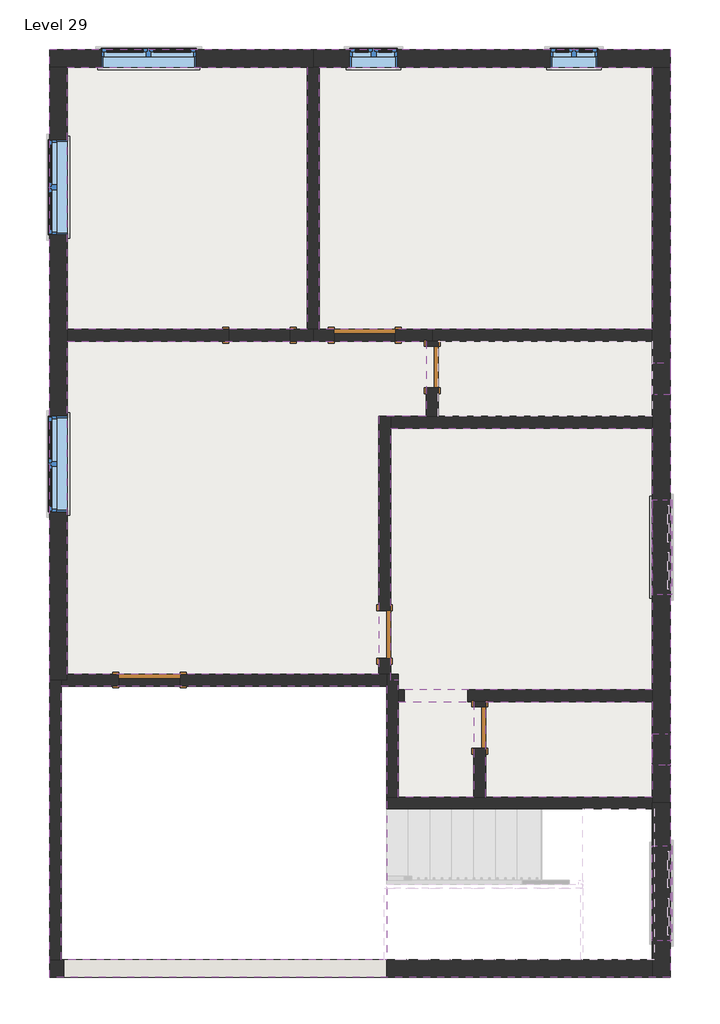
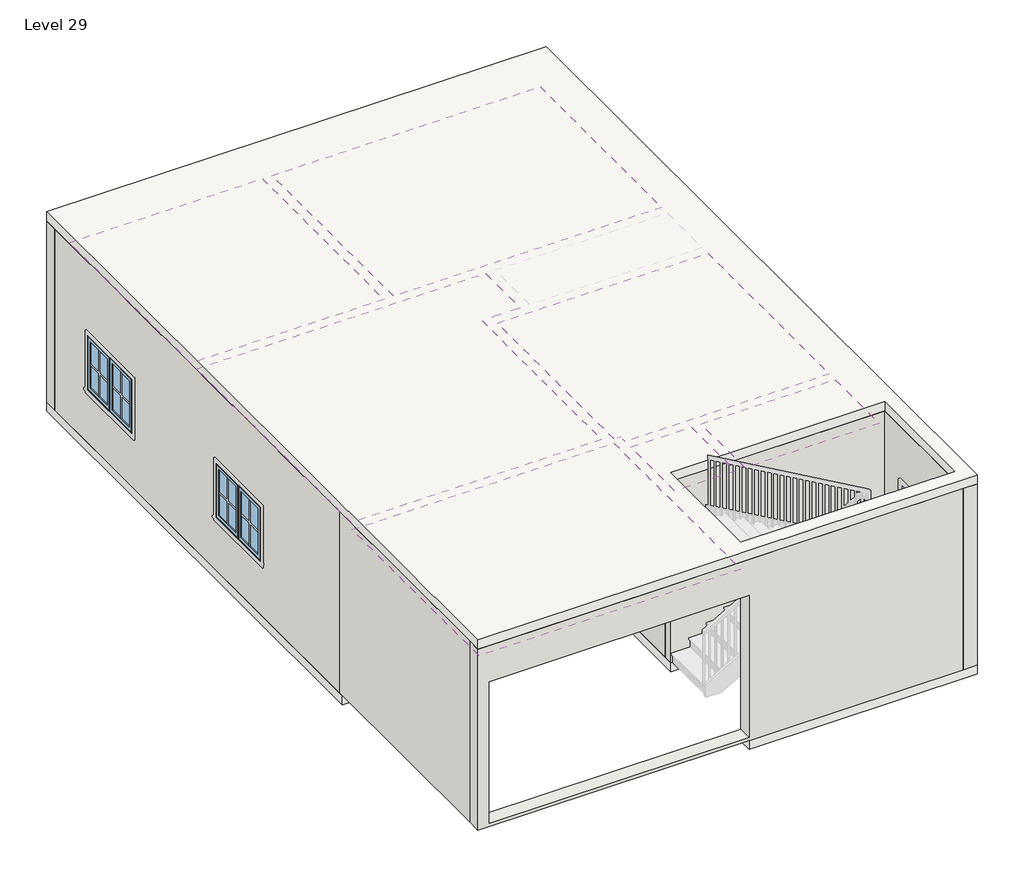
# One storey, part 1 of 2: 27 walls, 13 windows, 7 coverings, 6 doors, 2 slabs.
# Revit data of these elements (continued)
# Element 48 (IfcWindow, "Window-Casement-Double : 3'") (continued)
#   Frame Extension = 0' - 0 1/4"
#   Exterior Wall Closure = 0' - 1 1/4"
#   Interior Trim Visibility = yes
#   Exterior Trim Visibility = yes
#   Phase Created = New Construction
#   Materials on its faces: "Wood - Stained", "Glass", "Clad - White"
# Element 49 (IfcWindow, "Window-Casement-Double : 4'")
#   Mark = "131"
#   Window Inset = 0' - 0"
#   Interior Wall Closure = 0' - 2 1/4"
#   Frame Extension = 0' - 0 1/4"
#   Exterior Wall Closure = 0' - 1 1/4"
#   Interior Trim Visibility = yes
#   Exterior Trim Visibility = yes
#   Phase Created = New Construction
#   Materials on its faces: "Wood - Stained", "Glass", "Clad - White"
# Element 50 (IfcWindow, "Window-Casement-Double : 4'")
#   Mark = "132"
#   Window Inset = 0' - 0"
#   Interior Wall Closure = 0' - 2 1/4"
#   Frame Extension = 0' - 0 1/4"
#   Exterior Wall Closure = 0' - 1 1/4"
#   Interior Trim Visibility = yes
#   Exterior Trim Visibility = yes
#   Phase Created = New Construction
#   Materials on its faces: "Wood - Stained", "Glass", "Clad - White"
# Element 51 (IfcWindow, "Window-Casement-Double : 4'")
#   Mark = "133"
#   Window Inset = 0' - 0"
#   Interior Wall Closure = 0' - 2 1/4"
#   Frame Extension = 0' - 0 1/4"
#   Exterior Wall Closure = 0' - 1 1/4"
#   Interior Trim Visibility = yes
#   Exterior Trim Visibility = yes
#   Phase Created = New Construction
#   Materials on its faces: "Wood - Stained", "Glass", "Clad - White"
# Element 52 (IfcWindow, "Window-Casement-Double : 4'")
#   Mark = "134"
#   Window Inset = 0' - 0"
#   Interior Wall Closure = 0' - 2 1/4"
#   Frame Extension = 0' - 0 1/4"
#   Exterior Wall Closure = 0' - 1 1/4"
#   Interior Trim Visibility = yes
#   Exterior Trim Visibility = yes
#   Phase Created = New Construction
#   Materials on its faces: "Wood - Stained", "Glass", "Clad - White"
# Element 53 (IfcWindow, "Window-Casement-Double : 4'")
#   Mark = "135"
#   Window Inset = 0' - 0"
#   Interior Wall Closure = 0' - 2 1/4"
#   Frame Extension = 0' - 0 1/4"
#   Exterior Wall Closure = 0' - 1 1/4"
#   Interior Trim Visibility = yes
#   Exterior Trim Visibility = yes
#   Phase Created = New Construction
#   Materials on its faces: "Wood - Stained", "Glass", "Clad - White"
# Element 54 (IfcWindow, "Window-Casement-Double : 4'")
#   Mark = "140"
#   Window Inset = 0' - 0"
#   Interior Wall Closure = 0' - 2 1/4"
#   Frame Extension = 0' - 0 1/4"
#   Exterior Wall Closure = 0' - 1 1/4"
#   Interior Trim Visibility = yes
#   Exterior Trim Visibility = yes
#   Phase Created = New Construction
#   Materials on its faces: "Wood - Stained", "Glass", "Clad - White"
# Element 55 (IfcWindow, "Window-Casement-Double : 4'")
#   Mark = "141"
#   Window Inset = 0' - 0"
#   Interior Wall Closure = 0' - 2 1/4"
#   Frame Extension = 0' - 0 1/4"
#   Exterior Wall Closure = 0' - 1 1/4"
#   Interior Trim Visibility = yes
#   Exterior Trim Visibility = yes
#   Phase Created = New Construction
#   Materials on its faces: "Wood - Stained", "Glass", "Clad - White"
# Materials
#   "Default": colour RGB 127 127 127, transparency 0, Cost = 0
#   "Acoustic Ceiling Tile 24 x 48": class "Generic", colour RGB 229 229 229, transparency 0, Description = "Acoustic Ceiling Tile 24 x 48", Cost = 0
#   "Door - Panel": class "Wood", colour RGB 210 159 95, transparency 0, Cost = 0
#   "Door - Frame": colour RGB 118 70 51, transparency 0, Cost = 0
#   "Glass": class "Glass", colour RGB 0 128 192, transparency 0.75, Description = "Soda Lime Glass", Cost = 0
#   "Sash": class "Wood", colour RGB 224 178 126, transparency 0, Cost = 0
#   "Wood - Stained": class "Wood", colour RGB 224 178 126, transparency 0, Cost = 0
#   "Clad - White": class "Wood", colour RGB 242 242 238, transparency 0, Cost = 0
#   "Default Floor": colour RGB 128 128 128, transparency 0, Cost = 0
#   "TILE": class "Generic", colour RGB 120 120 120, transparency 0, Cost = 0
#   "Default Wall": colour RGB 128 128 128, transparency 0, Cost = 0
#   "WALL PAINT 4": class "Generic", colour RGB 120 120 120, transparency 0, Cost = 0
#   "MARBLE": class "Generic", colour RGB 120 120 120, transparency 0, Cost = 0
#   "WALL PAINT 5": class "Generic", colour RGB 120 120 120, transparency 0, Cost = 0
#   "WALL PAINT 2": class "Generic", colour RGB 120 120 120, transparency 0, Cost = 0
#   "WALL PAINT 3": class "Generic", colour RGB 120 120 120, transparency 0, Cost = 0
#   "WALL PAINT 1": class "Generic", colour RGB 120 120 120, transparency 0, Cost = 0
